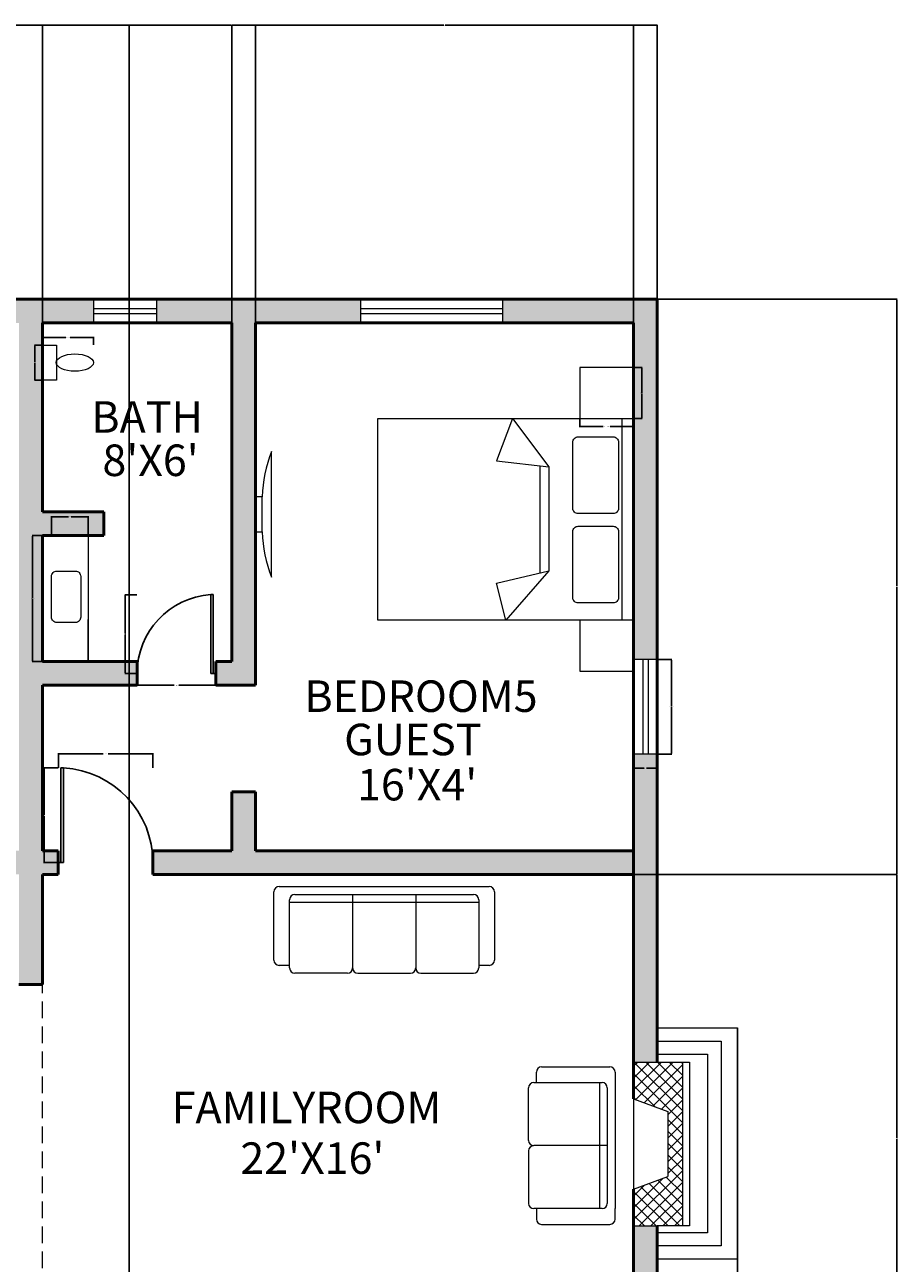
# Model space of a CAD drawing. Units: inches. Extents: x 2743 to 3669, y 1014 to 2282.
# Tile 5 of 5: x 3337 to 3669, y 1810 to 2282. Entities that reach past the tile are written whole.
import ezdxf

# ---------------------------------------------------------------- set-up
doc = ezdxf.new("R2010")
doc.units = ezdxf.units.IN
doc.linetypes.add('DASHED2', pattern=[9.525, 6.35, -3.175])
for name, color, linetype, lineweight in [('A-ANNO-DIMS', 2, 'Continuous', 18), ('A-AREA-IDEN', 4, 'Continuous', 18), ('A-DOOR', 211, 'Continuous', 25), ('A-EQPM', 51, 'Continuous', 18), ('A-FURN', 111, 'Continuous', 18), ('A-GLAZ', 40, 'Continuous', 20), ('A-GLAZ-PATT', 8, 'Continuous', 13), ('A-ROOF', 7, 'Continuous', 20), ('A-WALL', 7, 'Continuous', 50), ('A-WALL-OVHD', 8, 'DASHED2', 18)]:
    doc.layers.add(name, color=color, linetype=linetype, lineweight=lineweight)
doc.layers.add('A-FLOR-FIXT', color=11, linetype='Continuous', lineweight=18, true_color=0xee778f)
doc.layers.add('A-WALL-PATT', color=47, linetype='Continuous', lineweight=13, true_color=0x726c55)
doc.styles.get("Standard").update_dxf_attribs({"font": 'arial.ttf'})
doc.dimstyles.get("Standard").update_dxf_attribs({"dimtxt": 0.18, "dimasz": 0.18, "dimexe": 0.18, "dimexo": 0.0625, "dimgap": 0.09, "dimtad": 0, "dimtih": 1, "dimtoh": 1, "dimdec": 4, "dimzin": 0, "dimdsep": 46, "dimtxsty": 'Standard', "dimcen": 0.09, "dimadec": 0, "dimazin": 0, "dimtfac": 1, "dimtdec": 4, "dimtofl": 0, "dimtmove": 0, "dimatfit": 3, "dimfxl": 1, "dimtolj": 1, "dimtzin": 0, "dimarcsym": 0})

# ---------------------------------------------------------------- blocks, each defined once
blk = doc.blocks.new('DOOR-SINGLE-30IN')
for p, q in [((1, 0), (1, 30)), ((1, 30), (2, 30)), ((2, 30), (2, 0)), ((0, 0), (1, 0)), ((2, 0), (1, 0))]:
    blk.add_line(p, q)
blk.add_arc((0, 0.07), 30, 359.8725, 86.1776)
blk = doc.blocks.new('DOOR-SINGLE-36IN')
for p, q in [((1, 0), (1, 36)), ((1, 36), (2, 36)), ((2, 36), (2, 0)), ((0, 0), (1, 0)), ((2, 0), (1, 0))]:
    blk.add_line(p, q)
blk.add_arc((0, 0.06), 36, 359.9115, 86.8153)
blk = doc.blocks.new('WINDOW-24IN')
for p, q in [((0, 9), (0, 0)), ((0, 5.5), (24, 5.5)), ((24, 9), (24, 0)), ((0, 3.5), (24, 3.5))]:
    blk.add_line(p, q)
blk = doc.blocks.new('WINDOW-36IN')
for p, q in [((9, 36), (0, 36)), ((3.5, 36), (3.5, 0)), ((5.5, 36), (5.5, 0)), ((9, 0), (0, 0))]:
    blk.add_line(p, q)
blk = doc.blocks.new('BED-DOUBLE')
for p, q in [((4.31, 76.75), (4.31, 0)), ((32.31, 57.96), (48.69, 76.75)), ((48.69, 76.75), (52.23, 62.72)), ((52.23, 62.72), (32.31, 57.96)), ((32.31, 18.34), (32.31, 57.96)), ((35.7, 17.95), (35.72, 58.78)), ((46.06, 0), (32.31, 18.34)), ((52.23, 16.05), (32.31, 18.34)), ((46.06, 0), (52.23, 16.05))]:
    blk.add_line(p, q)
blk.add_lwpolyline([(0, 76.75), (97.38, 76.75), (97.38, 0), (0, 0)], close=True)
for points in [[(7.76, 70.21), (21.16, 70.21, -0.414214), (23.16, 68.21), (23.16, 43, -0.414214), (21.16, 41), (7.76, 41, -0.414214), (5.76, 43), (5.76, 68.21, -0.414214)], [(7.76, 36.18), (21.16, 36.18, -0.414214), (23.16, 34.18), (23.16, 8.97, -0.414214), (21.16, 6.97), (7.76, 6.97, -0.414214), (5.76, 8.97), (5.76, 34.18, -0.414214)]]:
    blk.add_lwpolyline(points, format="xyb", close=True)
blk = doc.blocks.new('NIGHTSTAND')
blk.add_lwpolyline([(0, 0), (20.5, 0), (20.5, 19.45), (0, 19.45)], close=True)
blk = doc.blocks.new('SOFA-TWO-SEAT')
for p, q in [((3, 54), (3, 58)), ((5, 60), (31, 60)), ((33, 58), (33, 6)), ((0, 32), (0, 52)), ((2, 54), (28, 54)), ((27, 54), (27, 6)), ((30, 52), (30, 8)), ((30, 30), (2, 30)), ((2, 30), (2, 30)), ((0, 28), (0, 8)), ((28, 6), (2, 6)), ((2, 6), (2, 6)), ((3, 6), (3, 2)), ((33, 2), (33, 6)), ((5, 0), (31, 0))]:
    blk.add_line(p, q)
for centre, start, end in [((5, 58), 90, 180), ((31, 58), 0, 90), ((2, 52), 90, 180), ((28, 52), 0, 90), ((2, 32), 180, 270), ((2, 28), 90, 180), ((2, 8), 180, 270), ((28, 8), 270, 0), ((5, 2), 180, 270), ((31, 2), 270, 0)]:
    blk.add_arc(centre, 2, start, end)
blk = doc.blocks.new('SOFA-THREE-SEAT')
for p, q in [((0, 5), (0, 31)), ((2, 33), (82, 33)), ((8, 30), (76, 30)), ((30, 30), (30, 2)), ((54, 30), (54, 2)), ((84, 31), (84, 5)), ((6, 2), (6, 28)), ((6, 27), (78, 27)), ((78, 28), (78, 2)), ((6, 3), (2, 3)), ((30, 2), (30, 2)), ((54, 2), (54, 2)), ((82, 3), (78, 3)), ((28, 0), (8, 0)), ((32, 0), (52, 0)), ((56, 0), (76, 0))]:
    blk.add_line(p, q)
for centre, start, end in [((2, 31), 90, 180), ((8, 28), 90, 180), ((76, 28), 0, 90), ((82, 31), 0, 90), ((2, 5), 180, 270), ((82, 5), 270, 0), ((8, 2), 180, 270), ((28, 2), 270, 0), ((32, 2), 180, 270), ((52, 2), 270, 0), ((56, 2), 180, 270), ((76, 2), 270, 0)]:
    blk.add_arc(centre, 2, start, end)
blk = doc.blocks.new('WC')
blk.add_lwpolyline([(0, 13.38), (5.3, 13.38), (5.3, 0), (0, 0)], close=True)
blk.add_ellipse((12.29, 6.69), major_axis=(7.08, 0), ratio=0.464281)
blk = doc.blocks.new('BASIN')
for p, q in [((13.95, 48), (13.95, 0)), ((13.95, 0), (13.95, 16.09))]:
    blk.add_line(p, q)
blk.add_lwpolyline([(2, 34.47), (9.09, 34.47, -0.414214), (11.09, 32.47), (11.09, 16.89, -0.414214), (9.09, 14.89), (2, 14.89, -0.414214), (0, 16.89), (0, 32.47, -0.414214)], format="xyb", close=True)
blk = doc.blocks.new('TV-SCREEN')
for p, q in [((6.11, 0), (6.11, 47.89)), ((2.64, 30.63), (0, 30.63)), ((2.64, 17.25), (2.64, 30.63)), ((0, 17.25), (2.64, 17.25))]:
    blk.add_line(p, q)
for centre, radius, start, end in [((54.67, 29.14), 52.05, 158.8899, 178.3579), ((54.74, 18.76), 52.13, 181.6646, 201.0965)]:
    blk.add_arc(centre, radius, start, end)
blk = doc.blocks.new('*D24')
at = {"layer": 'A-ANNO-DIMS', "color": 0, "lineweight": -2, "transparency": 16777216}
for p, q in [((3548.3, 2131.58), (3548.3, 2128.39)), ((3548.48, 2128.57), (3557.26, 2128.57)), ((3568.62, 2128.57), (3559.84, 2128.57)), ((3568.8, 2131.58), (3568.8, 2128.39))]:
    blk.add_line(p, q, dxfattribs=at)
at = {"layer": 'A-ANNO-DIMS', "color": 0, "transparency": 16777216}
for points in [[(3548.48, 2128.6), (3548.48, 2128.54), (3548.3, 2128.57)], [(3568.62, 2128.6), (3568.62, 2128.54), (3568.8, 2128.57)]]:
    blk.add_solid(points, dxfattribs=at)
at = {"layer": 'Defpoints', "color": 0, "transparency": 16777216}
for p in [(3548.3, 2131.64), (3568.8, 2131.64), (3548.3, 2128.57)]:
    blk.add_point(p, dxfattribs=at)
at = {"layer": 'A-ANNO-DIMS', "color": 0, "transparency": 16777216, "insert": (3558.55, 2128.57), "char_height": 0.18, "attachment_point": 5}
blk.add_mtext('\\A1;SIDE TABLE 20 TYP.', dxfattribs=at)
blk = doc.blocks.new('*D25')
at = {"layer": 'A-ANNO-DIMS', "color": 0, "lineweight": -2, "transparency": 16777216}
for p, q in [((3568.86, 2151.09), (3572.05, 2151.09)), ((3571.87, 2150.91), (3571.87, 2141.55)), ((3571.87, 2131.82), (3571.87, 2141.18)), ((3568.86, 2131.64), (3572.05, 2131.64))]:
    blk.add_line(p, q, dxfattribs=at)
at = {"layer": 'A-ANNO-DIMS', "color": 0, "transparency": 16777216}
for points in [[(3571.84, 2150.91), (3571.9, 2150.91), (3571.87, 2151.09)], [(3571.84, 2131.82), (3571.9, 2131.82), (3571.87, 2131.64)]]:
    blk.add_solid(points, dxfattribs=at)
at = {"layer": 'Defpoints', "color": 0, "transparency": 16777216}
for p in [(3568.8, 2151.09), (3568.8, 2131.64), (3571.87, 2131.64)]:
    blk.add_point(p, dxfattribs=at)
at = {"layer": 'A-ANNO-DIMS', "color": 0, "transparency": 16777216, "insert": (3571.87, 2141.37), "char_height": 0.18, "attachment_point": 5}
blk.add_mtext('\\A1;19 TYP.', dxfattribs=at)
blk = doc.blocks.new('*D26')
at = {"layer": 'A-ANNO-DIMS', "color": 0, "lineweight": -2, "transparency": 16777216}
for p, q in [((3379.76, 2034.53), (3379.76, 2029.91)), ((3409.8, 2034.53), (3409.8, 2029.91)), ((3379.94, 2030.09), (3393.84, 2030.09)), ((3409.62, 2030.09), (3395.71, 2030.09))]:
    blk.add_line(p, q, dxfattribs=at)
at = {"layer": 'A-ANNO-DIMS', "color": 0, "transparency": 16777216}
for points in [[(3379.94, 2030.12), (3379.94, 2030.06), (3379.76, 2030.09)], [(3409.62, 2030.12), (3409.62, 2030.06), (3409.8, 2030.09)]]:
    blk.add_solid(points, dxfattribs=at)
at = {"layer": 'Defpoints', "color": 0, "transparency": 16777216}
for p in [(3379.76, 2034.59), (3409.8, 2034.59), (3379.76, 2030.09)]:
    blk.add_point(p, dxfattribs=at)
at = {"layer": 'A-ANNO-DIMS', "color": 0, "transparency": 16777216, "insert": (3394.78, 2030.09), "char_height": 0.18, "attachment_point": 5}
blk.add_mtext('\\A1;DOOR 30 TYP.', dxfattribs=at)
blk = doc.blocks.new('*D27')
at = {"layer": 'A-ANNO-DIMS', "color": 0, "lineweight": -2, "transparency": 16777216}
for p, q in [((3379.7, 2064.59), (3375.08, 2064.59)), ((3375.26, 2064.41), (3375.26, 2049.78)), ((3375.26, 2034.77), (3375.26, 2049.41)), ((3379.7, 2034.59), (3375.08, 2034.59))]:
    blk.add_line(p, q, dxfattribs=at)
at = {"layer": 'A-ANNO-DIMS', "color": 0, "transparency": 16777216}
for points in [[(3375.23, 2064.41), (3375.29, 2064.41), (3375.26, 2064.59)], [(3375.23, 2034.77), (3375.29, 2034.77), (3375.26, 2034.59)]]:
    blk.add_solid(points, dxfattribs=at)
at = {"layer": 'Defpoints', "color": 0, "transparency": 16777216}
for p in [(3375.26, 2064.59), (3379.76, 2064.59), (3379.76, 2034.59)]:
    blk.add_point(p, dxfattribs=at)
at = {"layer": 'A-ANNO-DIMS', "color": 0, "transparency": 16777216, "insert": (3375.26, 2049.59), "char_height": 0.18, "attachment_point": 5}
blk.add_mtext('\\A1;30 TYP.', dxfattribs=at)
blk = doc.blocks.new('*D28')
at = {"layer": 'A-ANNO-DIMS', "color": 0, "lineweight": -2, "transparency": 16777216}
for p, q in [((3349.8, 1998.66), (3349.8, 2004.18)), ((3349.98, 2004), (3366.88, 2004)), ((3385.65, 2004), (3368.75, 2004)), ((3385.83, 1998.66), (3385.83, 2004.18))]:
    blk.add_line(p, q, dxfattribs=at)
at = {"layer": 'A-ANNO-DIMS', "color": 0, "transparency": 16777216}
for points in [[(3349.98, 2004.03), (3349.98, 2003.97), (3349.8, 2004)], [(3385.65, 2004.03), (3385.65, 2003.97), (3385.83, 2004)]]:
    blk.add_solid(points, dxfattribs=at)
at = {"layer": 'Defpoints', "color": 0, "transparency": 16777216}
for p in [(3385.83, 2004), (3349.8, 1998.59), (3385.83, 1998.59)]:
    blk.add_point(p, dxfattribs=at)
at = {"layer": 'A-ANNO-DIMS', "color": 0, "transparency": 16777216, "insert": (3367.81, 2004), "char_height": 0.18, "attachment_point": 5}
blk.add_mtext('\\A1;DOOR 36 TYP.', dxfattribs=at)
blk = doc.blocks.new('*D29')
at = {"layer": 'A-ANNO-DIMS', "color": 0, "lineweight": -2, "transparency": 16777216}
for p, q in [((3349.73, 1998.59), (3344.21, 1998.59)), ((3344.39, 1998.41), (3344.39, 1980.78)), ((3344.39, 1962.77), (3344.39, 1980.41)), ((3349.73, 1962.59), (3344.21, 1962.59))]:
    blk.add_line(p, q, dxfattribs=at)
at = {"layer": 'A-ANNO-DIMS', "color": 0, "transparency": 16777216}
for points in [[(3344.36, 1998.41), (3344.42, 1998.41), (3344.39, 1998.59)], [(3344.36, 1962.77), (3344.42, 1962.77), (3344.39, 1962.59)]]:
    blk.add_solid(points, dxfattribs=at)
at = {"layer": 'Defpoints', "color": 0, "transparency": 16777216}
for p in [(3344.39, 1998.59), (3349.8, 1998.59), (3349.8, 1962.59)]:
    blk.add_point(p, dxfattribs=at)
at = {"layer": 'A-ANNO-DIMS', "color": 0, "transparency": 16777216, "insert": (3344.39, 1980.59), "char_height": 0.18, "attachment_point": 5}
blk.add_mtext('\\A1;36 TYP.', dxfattribs=at)
blk = doc.blocks.new('*D40')
at = {"layer": 'A-ANNO-DIMS', "color": 0, "lineweight": -2, "transparency": 16777216}
for p, q in [((3343.8, 2159.71), (3343.8, 2162.74)), ((3343.98, 2162.56), (3352.71, 2162.56)), ((3362.99, 2162.56), (3354.26, 2162.56)), ((3363.17, 2159.71), (3363.17, 2162.74))]:
    blk.add_line(p, q, dxfattribs=at)
at = {"layer": 'A-ANNO-DIMS', "color": 0, "transparency": 16777216}
for points in [[(3343.98, 2162.59), (3343.98, 2162.53), (3343.8, 2162.56)], [(3362.99, 2162.59), (3362.99, 2162.53), (3363.17, 2162.56)]]:
    blk.add_solid(points, dxfattribs=at)
at = {"layer": 'Defpoints', "color": 0, "transparency": 16777216}
for p in [(3363.17, 2162.56), (3343.8, 2159.65), (3363.17, 2159.65)]:
    blk.add_point(p, dxfattribs=at)
at = {"layer": 'A-ANNO-DIMS', "color": 0, "transparency": 16777216, "insert": (3353.48, 2162.56), "char_height": 0.18, "attachment_point": 5}
blk.add_mtext('\\A1;WC 19 TYP.', dxfattribs=at)
blk = doc.blocks.new('*D41')
at = {"layer": 'A-ANNO-DIMS', "color": 0, "lineweight": -2, "transparency": 16777216}
for p, q in [((3343.73, 2159.65), (3340.71, 2159.65)), ((3340.89, 2159.47), (3340.89, 2153.14)), ((3340.89, 2146.45), (3340.89, 2152.78)), ((3343.73, 2146.27), (3340.71, 2146.27))]:
    blk.add_line(p, q, dxfattribs=at)
at = {"layer": 'A-ANNO-DIMS', "color": 0, "transparency": 16777216}
for points in [[(3340.86, 2159.47), (3340.92, 2159.47), (3340.89, 2159.65)], [(3340.86, 2146.45), (3340.92, 2146.45), (3340.89, 2146.27)]]:
    blk.add_solid(points, dxfattribs=at)
at = {"layer": 'Defpoints', "color": 0, "transparency": 16777216}
for p in [(3340.89, 2159.65), (3343.8, 2159.65), (3343.8, 2146.27)]:
    blk.add_point(p, dxfattribs=at)
at = {"layer": 'A-ANNO-DIMS', "color": 0, "transparency": 16777216, "insert": (3340.89, 2152.96), "char_height": 0.18, "attachment_point": 5}
blk.add_mtext('\\A1;13 TYP.', dxfattribs=at)
blk = doc.blocks.new('*D42')
at = {"layer": 'A-ANNO-DIMS', "color": 0, "lineweight": -2, "transparency": 16777216}
for p, q in [((3347.16, 2087.09), (3339.84, 2087.09)), ((3340.02, 2086.91), (3340.02, 2063.28)), ((3340.02, 2039.27), (3340.02, 2062.91)), ((3347.16, 2039.09), (3339.84, 2039.09))]:
    blk.add_line(p, q, dxfattribs=at)
at = {"layer": 'A-ANNO-DIMS', "color": 0, "transparency": 16777216}
for points in [[(3339.99, 2086.91), (3340.05, 2086.91), (3340.02, 2087.09)], [(3339.99, 2039.27), (3340.05, 2039.27), (3340.02, 2039.09)]]:
    blk.add_solid(points, dxfattribs=at)
at = {"layer": 'Defpoints', "color": 0, "transparency": 16777216}
for p in [(3340.02, 2087.09), (3347.22, 2087.09), (3347.22, 2039.09)]:
    blk.add_point(p, dxfattribs=at)
at = {"layer": 'A-ANNO-DIMS', "color": 0, "transparency": 16777216, "insert": (3340.02, 2063.09), "char_height": 0.18, "attachment_point": 5}
blk.add_mtext('\\A1;BASIN 48 TYP.', dxfattribs=at)
blk = doc.blocks.new('*D43')
at = {"layer": 'A-ANNO-DIMS', "color": 0, "lineweight": -2, "transparency": 16777216}
for p, q in [((3347.22, 2087.16), (3347.22, 2094.47)), ((3347.4, 2094.29), (3353.67, 2094.29)), ((3360.99, 2094.29), (3354.71, 2094.29)), ((3361.17, 2087.16), (3361.17, 2094.47))]:
    blk.add_line(p, q, dxfattribs=at)
at = {"layer": 'A-ANNO-DIMS', "color": 0, "transparency": 16777216}
for points in [[(3347.4, 2094.32), (3347.4, 2094.26), (3347.22, 2094.29)], [(3360.99, 2094.32), (3360.99, 2094.26), (3361.17, 2094.29)]]:
    blk.add_solid(points, dxfattribs=at)
at = {"layer": 'Defpoints', "color": 0, "transparency": 16777216}
for p in [(3361.17, 2094.29), (3347.22, 2087.09), (3361.17, 2087.09)]:
    blk.add_point(p, dxfattribs=at)
at = {"layer": 'A-ANNO-DIMS', "color": 0, "transparency": 16777216, "insert": (3354.19, 2094.29), "char_height": 0.18, "attachment_point": 5}
blk.add_mtext('\\A1;14 TYP.', dxfattribs=at)
blk = doc.blocks.new('*D48')
at = {"layer": 'A-ANNO-DIMS', "color": 0, "lineweight": -2, "transparency": 16777216}
for p, q in [((3577.86, 2039.89), (3583.38, 2039.89)), ((3583.2, 2039.71), (3583.2, 2022.07)), ((3583.2, 2004.07), (3583.2, 2021.7)), ((3577.86, 2003.89), (3583.38, 2003.89))]:
    blk.add_line(p, q, dxfattribs=at)
at = {"layer": 'A-ANNO-DIMS', "color": 0, "transparency": 16777216}
for points in [[(3583.17, 2039.71), (3583.23, 2039.71), (3583.2, 2039.89)], [(3583.17, 2004.07), (3583.23, 2004.07), (3583.2, 2003.89)]]:
    blk.add_solid(points, dxfattribs=at)
at = {"layer": 'Defpoints', "color": 0, "transparency": 16777216}
for p in [(3577.8, 2039.89), (3583.2, 2039.89), (3577.8, 2003.89)]:
    blk.add_point(p, dxfattribs=at)
at = {"layer": 'A-ANNO-DIMS', "color": 0, "transparency": 16777216, "insert": (3583.2, 2021.89), "char_height": 0.18, "attachment_point": 5}
blk.add_mtext('\\A1;WINDOW 36 TYP.', dxfattribs=at)
blk = doc.blocks.new('*D49')
at = {"layer": 'A-ANNO-DIMS', "color": 0, "lineweight": -2, "transparency": 16777216}
for p, q in [((3568.8, 2003.82), (3568.8, 1998.31)), ((3577.8, 2003.82), (3577.8, 1998.31)), ((3568.98, 1998.49), (3572.84, 1998.49)), ((3577.62, 1998.49), (3573.75, 1998.49))]:
    blk.add_line(p, q, dxfattribs=at)
at = {"layer": 'A-ANNO-DIMS', "color": 0, "transparency": 16777216}
for points in [[(3568.98, 1998.52), (3568.98, 1998.46), (3568.8, 1998.49)], [(3577.62, 1998.52), (3577.62, 1998.46), (3577.8, 1998.49)]]:
    blk.add_solid(points, dxfattribs=at)
at = {"layer": 'Defpoints', "color": 0, "transparency": 16777216}
for p in [(3568.8, 2003.89), (3577.8, 2003.89), (3577.8, 1998.49)]:
    blk.add_point(p, dxfattribs=at)
at = {"layer": 'A-ANNO-DIMS', "color": 0, "transparency": 16777216, "insert": (3573.3, 1998.49), "char_height": 0.18, "attachment_point": 5}
blk.add_mtext('\\A1;9 TYP.', dxfattribs=at)
blk = doc.blocks.new('*D62')
at = {"layer": 'A-ANNO-DIMS', "color": 0, "lineweight": -2, "transparency": 16777216}
for p, q in [((3608.38, 1899.55), (3608.38, 1014.41)), ((2803.91, 1765.52), (2803.91, 1014.41)), ((2804.09, 1014.59), (3205.75, 1014.59)), ((3608.2, 1014.59), (3206.54, 1014.59))]:
    blk.add_line(p, q, dxfattribs=at)
at = {"layer": 'A-ANNO-DIMS', "color": 0, "transparency": 16777216}
for points in [[(2804.09, 1014.62), (2804.09, 1014.56), (2803.91, 1014.59)], [(3608.2, 1014.62), (3608.2, 1014.56), (3608.38, 1014.59)]]:
    blk.add_solid(points, dxfattribs=at)
at = {"layer": 'Defpoints', "color": 0, "transparency": 16777216}
for p in [(3608.38, 1899.61), (2803.91, 1765.58), (3608.38, 1014.59)]:
    blk.add_point(p, dxfattribs=at)
at = {"layer": 'A-ANNO-DIMS', "color": 0, "transparency": 16777216, "insert": (3206.15, 1014.59), "char_height": 0.18, "attachment_point": 5}
blk.add_mtext('\\A1;804.5', dxfattribs=at)
blk = doc.blocks.new('*D65')
at = {"layer": 'A-ANNO-DIMS', "color": 0, "lineweight": -2, "transparency": 16777216}
for p, q in [((3013.8, 2168.16), (3013.8, 2281.6)), ((3013.98, 2281.42), (3214.5, 2281.42)), ((3415.62, 2281.42), (3215.09, 2281.42)), ((3415.8, 2168.16), (3415.8, 2281.6))]:
    blk.add_line(p, q, dxfattribs=at)
at = {"layer": 'A-ANNO-DIMS', "color": 0, "transparency": 16777216}
for points in [[(3013.98, 2281.45), (3013.98, 2281.39), (3013.8, 2281.42)], [(3415.62, 2281.45), (3415.62, 2281.39), (3415.8, 2281.42)]]:
    blk.add_solid(points, dxfattribs=at)
at = {"layer": 'Defpoints', "color": 0, "transparency": 16777216}
for p in [(3415.8, 2281.42), (3013.8, 2168.09), (3415.8, 2168.09)]:
    blk.add_point(p, dxfattribs=at)
at = {"layer": 'A-ANNO-DIMS', "color": 0, "transparency": 16777216, "insert": (3214.8, 2281.42), "char_height": 0.18, "attachment_point": 5}
blk.add_mtext('\\A1;402', dxfattribs=at)
blk = doc.blocks.new('*D66')
at = {"layer": 'A-ANNO-DIMS', "color": 0, "lineweight": -2, "transparency": 16777216}
for p, q in [((3415.8, 2168.16), (3415.8, 2281.6)), ((3415.98, 2281.42), (3496.52, 2281.42)), ((3577.62, 2281.42), (3497.08, 2281.42)), ((3577.8, 1899.67), (3577.8, 2281.6))]:
    blk.add_line(p, q, dxfattribs=at)
at = {"layer": 'A-ANNO-DIMS', "color": 0, "transparency": 16777216}
for points in [[(3415.98, 2281.45), (3415.98, 2281.39), (3415.8, 2281.42)], [(3577.62, 2281.45), (3577.62, 2281.39), (3577.8, 2281.42)]]:
    blk.add_solid(points, dxfattribs=at)
at = {"layer": 'Defpoints', "color": 0, "transparency": 16777216}
for p in [(3577.8, 2281.42), (3415.8, 2168.09), (3577.8, 1899.61)]:
    blk.add_point(p, dxfattribs=at)
at = {"layer": 'A-ANNO-DIMS', "color": 0, "transparency": 16777216, "insert": (3496.8, 2281.42), "char_height": 0.18, "attachment_point": 5}
blk.add_mtext('\\A1;162', dxfattribs=at)
blk = doc.blocks.new('*D69')
at = {"layer": 'A-ANNO-DIMS', "color": 0, "lineweight": -2, "transparency": 16777216}
for p, q in [((3568.86, 1958.09), (3669.11, 1958.09)), ((3668.93, 1957.91), (3668.93, 1857.78)), ((3668.93, 1757.27), (3668.93, 1857.41)), ((3568.86, 1757.09), (3669.11, 1757.09))]:
    blk.add_line(p, q, dxfattribs=at)
at = {"layer": 'A-ANNO-DIMS', "color": 0, "transparency": 16777216}
for points in [[(3668.9, 1957.91), (3668.96, 1957.91), (3668.93, 1958.09)], [(3668.9, 1757.27), (3668.96, 1757.27), (3668.93, 1757.09)]]:
    blk.add_solid(points, dxfattribs=at)
at = {"layer": 'Defpoints', "color": 0, "transparency": 16777216}
for p in [(3568.8, 1958.09), (3668.93, 1958.09), (3568.8, 1757.09)]:
    blk.add_point(p, dxfattribs=at)
at = {"layer": 'A-ANNO-DIMS', "color": 0, "transparency": 16777216, "insert": (3668.93, 1857.59), "char_height": 0.18, "attachment_point": 5}
blk.add_mtext('\\A1;201', dxfattribs=at)
blk = doc.blocks.new('*D70')
at = {"layer": 'A-ANNO-DIMS', "color": 0, "lineweight": -2, "transparency": 16777216}
for p, q in [((3577.86, 2177.09), (3669.11, 2177.09)), ((3668.93, 2176.91), (3668.93, 2067.78)), ((3668.93, 1958.27), (3668.93, 2067.41)), ((3568.86, 1958.09), (3669.11, 1958.09))]:
    blk.add_line(p, q, dxfattribs=at)
at = {"layer": 'A-ANNO-DIMS', "color": 0, "transparency": 16777216}
for points in [[(3668.9, 2176.91), (3668.96, 2176.91), (3668.93, 2177.09)], [(3668.9, 1958.27), (3668.96, 1958.27), (3668.93, 1958.09)]]:
    blk.add_solid(points, dxfattribs=at)
at = {"layer": 'Defpoints', "color": 0, "transparency": 16777216}
for p in [(3577.8, 2177.09), (3668.93, 2177.09), (3568.8, 1958.09)]:
    blk.add_point(p, dxfattribs=at)
at = {"layer": 'A-ANNO-DIMS', "color": 0, "transparency": 16777216, "insert": (3668.93, 2067.59), "char_height": 0.18, "attachment_point": 5}
blk.add_mtext('\\A1;219', dxfattribs=at)
blk = doc.blocks.new('*D71')
at = {"layer": 'A-ANNO-DIMS', "color": 0, "lineweight": -2, "transparency": 16777216}
for p, q in [((3343.8, 2168.16), (3343.8, 2281.6)), ((3343.98, 2281.42), (3379.58, 2281.42)), ((3415.62, 2281.42), (3380.01, 2281.42)), ((3415.8, 2168.16), (3415.8, 2281.6))]:
    blk.add_line(p, q, dxfattribs=at)
at = {"layer": 'A-ANNO-DIMS', "color": 0, "transparency": 16777216}
for points in [[(3343.98, 2281.45), (3343.98, 2281.39), (3343.8, 2281.42)], [(3415.62, 2281.45), (3415.62, 2281.39), (3415.8, 2281.42)]]:
    blk.add_solid(points, dxfattribs=at)
at = {"layer": 'Defpoints', "color": 0, "transparency": 16777216}
for p in [(3415.8, 2281.42), (3343.8, 2168.09), (3415.8, 2168.09)]:
    blk.add_point(p, dxfattribs=at)
at = {"layer": 'A-ANNO-DIMS', "color": 0, "transparency": 16777216, "insert": (3379.8, 2281.42), "char_height": 0.18, "attachment_point": 5}
blk.add_mtext('\\A1;72', dxfattribs=at)
blk = doc.blocks.new('*D72')
at = {"layer": 'A-ANNO-DIMS', "color": 0, "lineweight": -2, "transparency": 16777216}
for p, q in [((3424.8, 2168.16), (3424.8, 2281.6)), ((3424.98, 2281.42), (3496.52, 2281.42)), ((3568.62, 2281.42), (3497.08, 2281.42)), ((3568.8, 2168.16), (3568.8, 2281.6))]:
    blk.add_line(p, q, dxfattribs=at)
at = {"layer": 'A-ANNO-DIMS', "color": 0, "transparency": 16777216}
for points in [[(3424.98, 2281.45), (3424.98, 2281.39), (3424.8, 2281.42)], [(3568.62, 2281.45), (3568.62, 2281.39), (3568.8, 2281.42)]]:
    blk.add_solid(points, dxfattribs=at)
at = {"layer": 'Defpoints', "color": 0, "transparency": 16777216}
for p in [(3568.8, 2281.42), (3424.8, 2168.09), (3568.8, 2168.09)]:
    blk.add_point(p, dxfattribs=at)
at = {"layer": 'A-ANNO-DIMS', "color": 0, "transparency": 16777216, "insert": (3496.8, 2281.42), "char_height": 0.18, "attachment_point": 5}
blk.add_mtext('\\A1;144', dxfattribs=at)
blk = doc.blocks.new('*D78')
at = {"layer": 'A-ANNO-DIMS', "color": 0, "lineweight": -2, "transparency": 16777216}
for p, q in [((3271.8, 1130.9), (3271.8, 2281.6)), ((3271.98, 2281.42), (3323.82, 2281.42)), ((3376.57, 2281.42), (3324.73, 2281.42)), ((3376.75, 1130.9), (3376.75, 2281.6))]:
    blk.add_line(p, q, dxfattribs=at)
at = {"layer": 'A-ANNO-DIMS', "color": 0, "transparency": 16777216}
for points in [[(3271.98, 2281.45), (3271.98, 2281.39), (3271.8, 2281.42)], [(3376.57, 2281.45), (3376.57, 2281.39), (3376.75, 2281.42)]]:
    blk.add_solid(points, dxfattribs=at)
at = {"layer": 'Defpoints', "color": 0, "transparency": 16777216}
for p in [(3376.75, 2281.42), (3271.8, 1130.83), (3376.75, 1130.83)]:
    blk.add_point(p, dxfattribs=at)
at = {"layer": 'A-ANNO-DIMS', "color": 0, "transparency": 16777216, "insert": (3324.27, 2281.42), "char_height": 0.18, "attachment_point": 5}
blk.add_mtext('\\A1;104.95', dxfattribs=at)

msp = doc.modelspace()

# ---------------------------------------------------------------- hatches: boundary and pattern name
at = {"layer": 'A-GLAZ-PATT'}
h = msp.add_hatch(dxfattribs=at)
h.set_pattern_fill('ANSI37', color=256)
h.paths.add_polyline_path([(3587.373, 1886.608), (3577.796, 1886.608), (3568.796, 1886.608), (3568.796, 1872.608), (3581.802, 1867.739), (3581.802, 1843.047), (3568.796, 1838.222), (3568.796, 1824.222), (3577.796, 1824.222), (3587.373, 1824.222)])
at = {"layer": 'A-WALL-PATT'}
h = msp.add_hatch(color=256, dxfattribs=at)
h.dxf.hatch_style = 1
h.paths.add_polyline_path([(3334.796, 2168.094), (3334.796, 1967.094), (3328.796, 1967.094), (3328.796, 1958.094), (3334.796, 1958.094), (3334.796, 1916.094), (3343.796, 1916.094), (3343.796, 1958.094), (3349.796, 1958.094), (3349.796, 1967.094), (3343.796, 1967.094), (3343.796, 2030.094), (3379.796, 2030.094), (3379.796, 2039.094), (3343.796, 2039.094), (3343.796, 2087.094), (3367.124, 2087.094), (3367.124, 2096.094), (3343.796, 2096.094), (3343.796, 2168.094), (3363.161, 2168.094), (3363.161, 2177.094), (3268.796, 2177.094), (3268.796, 2168.094)])
h = msp.add_hatch(color=256, dxfattribs=at)
h.dxf.hatch_style = 1
h.paths.add_polyline_path([(3387.161, 2177.094), (3387.161, 2168.094), (3415.796, 2168.094), (3415.796, 2039.094), (3409.796, 2039.094), (3409.796, 2030.094), (3424.796, 2030.094), (3424.796, 2168.094), (3465.008, 2168.094), (3465.008, 2177.094)])
h = msp.add_hatch(color=256, dxfattribs=at)
h.dxf.hatch_style = 1
h.paths.add_polyline_path([(3568.796, 2168.094), (3568.796, 2039.886), (3577.796, 2039.886), (3577.796, 2177.094), (3519.008, 2177.094), (3519.008, 2168.094)])
h = msp.add_hatch(color=256, dxfattribs=at)
h.dxf.hatch_style = 1
h.paths.add_polyline_path([(3577.796, 2003.886), (3568.796, 2003.886), (3568.796, 1886.608), (3577.796, 1886.608), (3577.796, 1889.608), (3577.796, 1894.608), (3577.796, 1899.608)])
h = msp.add_hatch(color=256, dxfattribs=at)
h.dxf.hatch_style = 1
h.paths.add_polyline_path([(3568.796, 1967.094), (3424.796, 1967.094), (3424.796, 1989.532), (3415.796, 1989.532), (3415.796, 1967.094), (3385.796, 1967.094), (3385.796, 1958.094), (3568.796, 1958.094)])
h = msp.add_hatch(color=256, dxfattribs=at)
h.dxf.hatch_style = 1
h.paths.add_polyline_path([(3415.796, 1757.094), (3415.796, 1565.094), (3424.796, 1565.094), (3424.796, 1679.094), (3430.796, 1679.094), (3430.796, 1685.094), (3424.796, 1685.094), (3424.796, 1757.094), (3472.796, 1757.094), (3472.796, 1721.094), (3478.796, 1721.094), (3478.796, 1757.094), (3568.796, 1757.094), (3568.796, 1732.183), (3577.796, 1732.183), (3577.796, 1824.222), (3568.796, 1824.222), (3568.796, 1766.094), (3396.681, 1766.094), (3396.681, 1757.094)])

# ---------------------------------------------------------------- linework, layer by layer
at = {"layer": 'A-GLAZ'}
for p, q in [((3465.008, 2168.094), (3465.008, 2177.094)), ((3519.008, 2168.094), (3519.008, 2177.094)), ((3465.008, 2173.594), (3519.008, 2173.594)), ((3465.008, 2171.594), (3519.008, 2171.594)), ((3568.796, 1886.608), (3577.796, 1886.608)), ((3577.796, 1886.608), (3590.005, 1886.608)), ((3587.373, 1886.608), (3587.373, 1824.222)), ((3590.005, 1886.608), (3590.005, 1824.222)), ((3568.796, 1872.608), (3581.802, 1867.739)), ((3568.796, 1872.608), (3568.796, 1838.222)), ((3581.802, 1867.739), (3581.802, 1843.047)), ((3568.796, 1838.222), (3581.802, 1843.047)), ((3568.796, 1824.222), (3577.796, 1824.222)), ((3590.005, 1824.222), (3577.796, 1824.222))]:
    msp.add_line(p, q, dxfattribs=at)
at = {"layer": 'A-ROOF'}
for p, q in [((3577.796, 1894.608), (3577.796, 1899.608)), ((3577.796, 1899.608), (3608.383, 1899.608)), ((3608.383, 1899.608), (3608.383, 1811.608)), ((3577.796, 1889.608), (3577.796, 1894.608)), ((3577.796, 1894.608), (3602.064, 1894.608)), ((3602.064, 1894.608), (3602.064, 1816.608)), ((3577.796, 1886.608), (3577.796, 1889.608)), ((3577.796, 1889.608), (3596.891, 1889.608)), ((3596.891, 1889.608), (3596.891, 1821.608)), ((3596.891, 1821.608), (3577.796, 1821.608)), ((3602.064, 1816.608), (3577.796, 1816.608)), ((3608.383, 1811.608), (3577.796, 1811.608))]:
    msp.add_line(p, q, dxfattribs=at)
at = {"layer": 'A-WALL'}
for p, q in [((3343.796, 2096.094), (3343.796, 2168.094)), ((3343.796, 2168.094), (3415.796, 2168.094)), ((3415.796, 2039.094), (3415.796, 2168.094)), ((3424.796, 2030.094), (3424.796, 2168.094)), ((3424.796, 2168.094), (3568.796, 2168.094)), ((3568.796, 2168.094), (3568.796, 1872.608)), ((3343.796, 2096.094), (3367.124, 2096.094)), ((3367.124, 2096.094), (3367.124, 2087.094)), ((3343.796, 2087.094), (3367.124, 2087.094)), ((3343.796, 2039.094), (3343.796, 2087.094)), ((3343.796, 2039.094), (3379.796, 2039.094)), ((3379.796, 2039.094), (3379.796, 2030.094)), ((3409.796, 2039.094), (3409.796, 2030.094)), ((3409.796, 2039.094), (3415.796, 2039.094)), ((3343.796, 2030.094), (3379.796, 2030.094)), ((3343.796, 1967.094), (3343.796, 2030.094)), ((3409.796, 2030.094), (3424.796, 2030.094)), ((3415.796, 1989.532), (3424.796, 1989.532)), ((3415.796, 1967.094), (3415.796, 1989.532)), ((3424.796, 1967.094), (3424.796, 1989.532)), ((3343.796, 1967.094), (3349.796, 1967.094)), ((3349.796, 1967.094), (3349.796, 1958.094)), ((3385.796, 1967.094), (3385.796, 1958.094)), ((3385.796, 1967.094), (3415.796, 1967.094)), ((3424.796, 1967.094), (3568.796, 1967.094)), ((3343.796, 1916.094), (3343.796, 1958.094)), ((3343.796, 1958.094), (3349.796, 1958.094)), ((3385.796, 1958.094), (3568.796, 1958.094)), ((3334.796, 1916.094), (3343.796, 1916.094)), ((3568.796, 1838.222), (3568.796, 1766.094))]:
    msp.add_line(p, q, dxfattribs=at)
for points in [[(3268.796, 2177.094), (3577.796, 2177.094), (3577.796, 1886.608)], [(3577.796, 1824.222), (3577.796, 1372.069)]]:
    msp.add_lwpolyline(points, dxfattribs=at)
at = {"layer": 'A-WALL-OVHD'}
msp.add_line((3343.796, 1808.094), (3343.796, 1916.094), dxfattribs=at)

# ---------------------------------------------------------------- block references
at = {"layer": 'A-DOOR', "extrusion": (0, 0, -1), "zscale": -1}
msp.add_blockref('DOOR-SINGLE-30IN', (-3409.797, 2034.594), dxfattribs=at)
at = {"layer": 'A-DOOR'}
msp.add_blockref('DOOR-SINGLE-36IN', (3349.796, 1962.594), dxfattribs=at)
at = {"layer": 'A-EQPM'}
msp.add_blockref('TV-SCREEN', (3424.796, 2071.256), dxfattribs=at)
at = {"layer": 'A-FLOR-FIXT'}
for name, p in [('WC', (3343.796, 2146.269)), ('BASIN', (3347.218, 2039.094))]:
    msp.add_blockref(name, p, dxfattribs=at)
at = {"layer": 'A-FURN', "rotation": 180}
for name, p in [('NIGHTSTAND', (3568.797, 2151.09)), ('BED-DOUBLE', (3568.797, 2131.643)), ('NIGHTSTAND', (3568.797, 2054.894))]:
    msp.add_blockref(name, p, dxfattribs=at)
at = {"layer": 'A-FURN'}
for name, p in [('SOFA-THREE-SEAT', (3431.832, 1920.446)), ('SOFA-TWO-SEAT', (3528.78, 1824.804))]:
    msp.add_blockref(name, p, dxfattribs=at)
at = {"layer": 'A-GLAZ'}
for name, p in [('WINDOW-24IN', (3363.161, 2168.094)), ('WINDOW-36IN', (3568.796, 2003.886))]:
    msp.add_blockref(name, p, dxfattribs=at)

# ---------------------------------------------------------------- texts
at = {"layer": 'A-AREA-IDEN'}
for tag, p in [('BATH', (3362.364, 2126.262)), ("8'X6'", (3366.578, 2109.769)), ('BEDROOM5', (3443.493, 2019.937)), ('GUEST', (3458.595, 2003.445)), ("16'X4'", (3463.512, 1986.25)), ('FAMILYROOM', (3392.967, 1863.338)), ("22'X16'", (3419.089, 1844.031))]:
    msp.add_attdef(tag, p, '', height=12, dxfattribs=at)

# ---------------------------------------------------------------- dimensions: what is measured, and where the dimension line sits
at = {"layer": 'A-ANNO-DIMS'}
for base, p1, p2, override, picture, middle in [((3415.796, 2281.421), (3013.796, 2168.094), (3415.796, 2168.094), {"dimdec": 0, "dimlfac": 1, "dimrnd": 0, "dimzin": 0, "dimdsep": 46, "dimlunit": 2}, '*D65', (3214.796, 2281.421)), ((3376.7513, 2281.4212), (3271.7965, 1130.8347), (3376.7513, 1130.8347), {"dimdec": 2, "dimlfac": 1, "dimrnd": 0, "dimzin": 0, "dimdsep": 46, "dimlunit": 2}, '*D78', (3324.2739, 2281.4212)), ((3415.796, 2281.421), (3343.796, 2168.094), (3415.796, 2168.094), {"dimdec": 0, "dimlfac": 1, "dimrnd": 0, "dimzin": 0, "dimdsep": 46, "dimlunit": 2}, '*D71', (3379.796, 2281.421)), ((3577.796, 2281.421), (3415.796, 2168.094), (3577.796, 1899.608), {"dimdec": 0, "dimlfac": 1, "dimrnd": 0, "dimzin": 0, "dimdsep": 46, "dimlunit": 2}, '*D66', (3496.796, 2281.421)), ((3568.796, 2281.421), (3424.796, 2168.094), (3568.796, 2168.094), {"dimdec": 0, "dimlfac": 1, "dimrnd": 0, "dimzin": 0, "dimdsep": 46, "dimlunit": 2}, '*D72', (3496.796, 2281.421)), ((3608.383, 1014.589), (2803.91, 1765.581), (3608.383, 1899.608), {"dimdec": 1, "dimlfac": 1, "dimrnd": 0, "dimzin": 0, "dimdsep": 46, "dimlunit": 2}, '*D62', (3206.146, 1014.589))]:
    dim = msp.add_linear_dim(base=base, p1=p1, p2=p2, dimstyle='Standard', override=override, dxfattribs=at)
    dim.commit()
    dim.dimension.update_dxf_attribs({"geometry": picture, "text_midpoint": middle})
for base, p1, p2, picture, middle in [((3668.933, 2177.094), (3568.796, 1958.094), (3577.796, 2177.094), '*D70', (3668.933, 2067.594)), ((3668.933, 1958.094), (3568.796, 1757.094), (3568.796, 1958.094), '*D69', (3668.933, 1857.594))]:
    dim = msp.add_linear_dim(base=base, p1=p1, p2=p2, angle=90, dimstyle='Standard', override={"dimdec": 0, "dimlfac": 1, "dimrnd": 0, "dimzin": 0, "dimdsep": 46, "dimlunit": 2}, dxfattribs=at)
    dim.commit()
    dim.dimension.update_dxf_attribs({"geometry": picture, "text_midpoint": middle})
for base, p1, p2, text, picture, middle in [((3363.171, 2162.557), (3343.796, 2159.651), (3363.171, 2159.651), 'WC <> TYP.', '*D40', (3353.484, 2162.557)), ((3361.169, 2094.294), (3347.218, 2087.094), (3361.169, 2087.094), '<> TYP.', '*D43', (3354.193, 2094.294)), ((3385.826, 2003.999), (3349.796, 1998.594), (3385.826, 1998.594), 'DOOR <> TYP.', '*D28', (3367.811, 2003.999)), ((3577.796, 1998.486), (3568.796, 2003.886), (3577.796, 2003.886), '<> TYP.', '*D49', (3573.296, 1998.486))]:
    dim = msp.add_linear_dim(base=base, p1=p1, p2=p2, text=text, dimstyle='Standard', override={"dimdec": 0, "dimlfac": 1, "dimrnd": 0, "dimzin": 0, "dimdsep": 46, "dimlunit": 2}, dxfattribs=at)
    dim.commit()
    dim.dimension.update_dxf_attribs({"geometry": picture, "text_midpoint": middle})
for base, p1, p2, angle, text, picture, middle in [((3340.89, 2159.651), (3343.796, 2146.269), (3343.796, 2159.651), 90, '<> TYP.', '*D41', (3340.89, 2152.96)), ((3571.871, 2131.643), (3568.796, 2151.091), (3568.796, 2131.643), 270, '<> TYP.', '*D25', (3571.871, 2141.367)), ((3548.302, 2128.569), (3568.796, 2131.643), (3548.302, 2131.643), 180, 'SIDE TABLE <> TYP.', '*D24', (3558.549, 2128.569)), ((3340.018, 2087.094), (3347.218, 2039.094), (3347.218, 2087.094), 90, 'BASIN <> TYP.', '*D42', (3340.018, 2063.094)), ((3375.256, 2064.594), (3379.761, 2034.594), (3379.761, 2064.594), 90, '<> TYP.', '*D27', (3375.256, 2049.594)), ((3583.196, 2039.886), (3577.796, 2003.886), (3577.796, 2039.886), 90, 'WINDOW <> TYP.', '*D48', (3583.196, 2021.886)), ((3379.761, 2030.089), (3409.796, 2034.594), (3379.761, 2034.594), 180, 'DOOR <> TYP.', '*D26', (3394.779, 2030.089)), ((3344.392, 1998.594), (3349.796, 1962.594), (3349.796, 1998.594), 90, '<> TYP.', '*D29', (3344.392, 1980.594))]:
    dim = msp.add_linear_dim(base=base, p1=p1, p2=p2, angle=angle, text=text, dimstyle='Standard', override={"dimdec": 0, "dimlfac": 1, "dimrnd": 0, "dimzin": 0, "dimdsep": 46, "dimlunit": 2}, dxfattribs=at)
    dim.commit()
    dim.dimension.update_dxf_attribs({"geometry": picture, "text_midpoint": middle})

doc.saveas('drawing.dxf')
